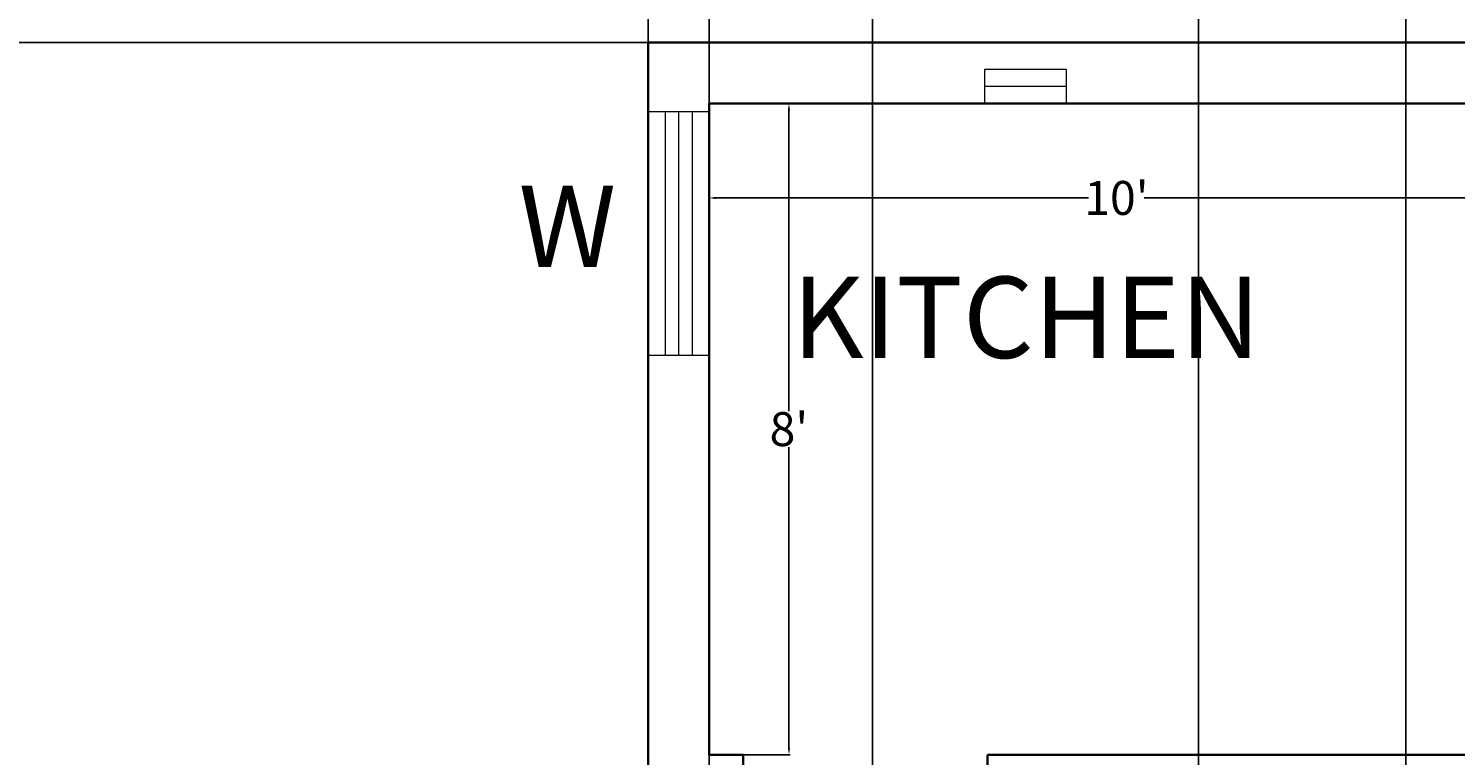
# Model space of a CAD drawing. Units: inches. Extents: x -304 to 580, y 363 to 1149.
# Tile 9 of 11: x -114 to 96, y 900 to 1007. Entities that reach past the tile are written whole.
import ezdxf

# ---------------------------------------------------------------- set-up
doc = ezdxf.new("R2010")
doc.units = ezdxf.units.IN
doc.header["$MEASUREMENT"] = 0
for name, color, linetype, lineweight in [('A-ANNO-DIMS', 2, 'Continuous', 13), ('A-ANNO-IDEN', 7, 'Continuous', 18), ('A-AREA-IDEN', 7, 'Continuous', 25), ('A-GLAZ', 4, 'Continuous', 18), ('A-GLAZ-VENT', 4, 'Continuous', 18), ('A-WALL', 40, 'Continuous', 35)]:
    doc.layers.add(name, color=color, linetype=linetype, lineweight=lineweight)
doc.styles.get("Standard").update_dxf_attribs({"font": 'arial.ttf'})
doc.dimstyles.get("Standard").update_dxf_attribs({"dimtxt": 1, "dimasz": 1, "dimexe": 0.18, "dimexo": 0.0625, "dimgap": 0.09, "dimtad": 0, "dimtih": 1, "dimtoh": 1, "dimdec": 0, "dimzin": 0, "dimdsep": 46, "dimlunit": 3, "dimtxsty": 'Standard', "dimcen": 0.09, "dimadec": 0, "dimazin": 0, "dimtfac": 1, "dimtdec": 0, "dimtofl": 0, "dimtmove": 0, "dimatfit": 3, "dimfxl": 1, "dimtolj": 1, "dimtzin": 0, "dimarcsym": 0})

# ---------------------------------------------------------------- blocks, each defined once
blk = doc.blocks.new('*D1')
at = {"layer": 'A-ANNO-DIMS', "color": 0, "lineweight": -2, "transparency": 16777216}
for p, q in [((-22.63, 1004.95), (-237.62, 1004.95)), ((-237.44, 1003.95), (-237.44, 721.93)), ((-237.44, 402.95), (-237.44, 684.96)), ((-22.63, 401.95), (-237.62, 401.95))]:
    blk.add_line(p, q, dxfattribs=at)
at = {"layer": 'A-ANNO-DIMS', "color": 0, "transparency": 16777216}
for points in [[(-237.61, 1003.95), (-237.28, 1003.95), (-237.44, 1004.95)], [(-237.61, 402.95), (-237.28, 402.95), (-237.44, 401.95)]]:
    blk.add_solid(points, dxfattribs=at)
at = {"layer": 'Defpoints', "color": 0, "transparency": 16777216}
for p in [(-22.57, 1004.95), (-237.44, 401.95), (-22.57, 401.95)]:
    blk.add_point(p, dxfattribs=at)
at = {"layer": 'A-ANNO-DIMS', "color": 0, "transparency": 16777216, "insert": (-237.44, 703.45), "char_height": 1, "attachment_point": 5}
blk.add_mtext('\\A1;{\\H36x;50\'-3"}', dxfattribs=at)
blk = doc.blocks.new('*D2')
at = {"layer": 'A-ANNO-DIMS', "color": 0, "lineweight": -2, "transparency": 16777216}
for p, q in [((-22.57, 1005.01), (-22.57, 1060.38)), ((-21.57, 1060.2), (84.7, 1060.2)), ((315.43, 1060.2), (209.16, 1060.2)), ((316.43, 1005.01), (316.43, 1060.38))]:
    blk.add_line(p, q, dxfattribs=at)
at = {"layer": 'A-ANNO-DIMS', "color": 0, "transparency": 16777216}
for points in [[(-21.57, 1060.37), (-21.57, 1060.04), (-22.57, 1060.2)], [(315.43, 1060.37), (315.43, 1060.04), (316.43, 1060.2)]]:
    blk.add_solid(points, dxfattribs=at)
at = {"layer": 'Defpoints', "color": 0, "transparency": 16777216}
for p in [(316.43, 1060.2), (-22.57, 1004.95), (316.43, 1004.95)]:
    blk.add_point(p, dxfattribs=at)
at = {"layer": 'A-ANNO-DIMS', "color": 0, "transparency": 16777216, "insert": (146.93, 1060.2), "char_height": 1, "attachment_point": 5}
blk.add_mtext('\\A1;{\\H36x;28\'-3"}', dxfattribs=at)
blk = doc.blocks.new('*D5')
at = {"layer": 'A-ANNO-DIMS', "color": 0, "lineweight": -2, "transparency": 16777216}
for p, q in [((-13.57, 995.88), (-13.57, 981.84)), ((106.43, 995.88), (106.43, 981.84)), ((-12.57, 982.02), (42.33, 982.02)), ((105.43, 982.02), (50.53, 982.02))]:
    blk.add_line(p, q, dxfattribs=at)
at = {"layer": 'A-ANNO-DIMS', "color": 0, "transparency": 16777216}
for points in [[(-12.57, 982.19), (-12.57, 981.85), (-13.57, 982.02)], [(105.43, 982.19), (105.43, 981.85), (106.43, 982.02)]]:
    blk.add_solid(points, dxfattribs=at)
at = {"layer": 'Defpoints', "color": 0, "transparency": 16777216}
for p in [(-13.57, 995.95), (106.43, 995.95), (106.43, 982.02)]:
    blk.add_point(p, dxfattribs=at)
at = {"layer": 'A-ANNO-DIMS', "color": 0, "transparency": 16777216, "insert": (46.43, 982.02), "char_height": 1, "attachment_point": 5}
blk.add_mtext("\\A1;{\\H5x;10'}", dxfattribs=at)
blk = doc.blocks.new('*D6')
at = {"layer": 'A-ANNO-DIMS', "color": 0, "lineweight": -2, "transparency": 16777216}
for p, q in [((-13.51, 995.95), (-1.64, 995.95)), ((-1.82, 994.95), (-1.82, 950.59)), ((-1.82, 900.95), (-1.82, 945.3)), ((-13.51, 899.95), (-1.64, 899.95))]:
    blk.add_line(p, q, dxfattribs=at)
at = {"layer": 'A-ANNO-DIMS', "color": 0, "transparency": 16777216}
for points in [[(-1.98, 994.95), (-1.65, 994.95), (-1.82, 995.95)], [(-1.98, 900.95), (-1.65, 900.95), (-1.82, 899.95)]]:
    blk.add_solid(points, dxfattribs=at)
at = {"layer": 'Defpoints', "color": 0, "transparency": 16777216}
for p in [(-13.57, 995.95), (-13.57, 899.95), (-1.82, 899.95)]:
    blk.add_point(p, dxfattribs=at)
at = {"layer": 'A-ANNO-DIMS', "color": 0, "transparency": 16777216, "insert": (-1.82, 947.95), "char_height": 1, "attachment_point": 5}
blk.add_mtext("\\A1;{\\H5x;8'}", dxfattribs=at)
blk = doc.blocks.new('WIN-36IN')
for p, q in [((0, 6.5), (36, 6.5)), ((0, 4.5), (36, 4.5)), ((0, 2.5), (36, 2.5))]:
    blk.add_line(p, q)
blk.add_lwpolyline([(0, 0), (0, 9), (36, 9), (36, 0)], close=True)
blk = doc.blocks.new('VENT-12IN')
blk.add_line((0, 2.5), (12, 2.5))
blk.add_lwpolyline([(0, 0), (0, 5), (12, 5), (12, 0)], close=True)
blk = doc.blocks.new('*D34')
at = {"layer": 'A-ANNO-DIMS', "color": 0, "lineweight": -2, "transparency": 16777216}
for p, q in [((10.51, 550.01), (10.51, 1042.88)), ((11.51, 1042.7), (33.07, 1042.7)), ((57.51, 1042.7), (35.95, 1042.7)), ((58.51, 550.01), (58.51, 1042.88))]:
    blk.add_line(p, q, dxfattribs=at)
at = {"layer": 'A-ANNO-DIMS', "color": 0, "transparency": 16777216}
for points in [[(11.51, 1042.86), (11.51, 1042.53), (10.51, 1042.7)], [(57.51, 1042.86), (57.51, 1042.53), (58.51, 1042.7)]]:
    blk.add_solid(points, dxfattribs=at)
at = {"layer": 'Defpoints', "color": 0, "transparency": 16777216}
for p in [(58.51, 1042.7), (10.51, 549.95), (58.51, 549.95)]:
    blk.add_point(p, dxfattribs=at)
at = {"layer": 'A-ANNO-DIMS', "color": 0, "transparency": 16777216, "insert": (34.51, 1042.7), "char_height": 1, "attachment_point": 5}
blk.add_mtext('\\A1;4\'-0"', dxfattribs=at)
blk = doc.blocks.new('*D35')
at = {"layer": 'A-ANNO-DIMS', "color": 0, "lineweight": -2, "transparency": 16777216}
for p, q in [((-13.57, 550.01), (-13.57, 1042.88)), ((-12.57, 1042.7), (-2.96, 1042.7)), ((9.51, 1042.7), (-0.1, 1042.7)), ((10.51, 550.01), (10.51, 1042.88))]:
    blk.add_line(p, q, dxfattribs=at)
at = {"layer": 'A-ANNO-DIMS', "color": 0, "transparency": 16777216}
for points in [[(-12.57, 1042.86), (-12.57, 1042.53), (-13.57, 1042.7)], [(9.51, 1042.86), (9.51, 1042.53), (10.51, 1042.7)]]:
    blk.add_solid(points, dxfattribs=at)
at = {"layer": 'Defpoints', "color": 0, "transparency": 16777216}
for p in [(10.51, 1042.7), (-13.57, 549.95), (10.51, 549.95)]:
    blk.add_point(p, dxfattribs=at)
at = {"layer": 'A-ANNO-DIMS', "color": 0, "transparency": 16777216, "insert": (-1.53, 1042.7), "char_height": 1, "attachment_point": 5}
blk.add_mtext('\\A1;2\'-0"', dxfattribs=at)
blk = doc.blocks.new('*D36')
at = {"layer": 'A-ANNO-DIMS', "color": 0, "lineweight": -2, "transparency": 16777216}
for p, q in [((-22.57, 516.57), (-22.57, 1042.88)), ((-21.57, 1042.7), (30.65, 1042.7)), ((88.04, 1042.7), (35.82, 1042.7)), ((89.04, 516.57), (89.04, 1042.88))]:
    blk.add_line(p, q, dxfattribs=at)
at = {"layer": 'A-ANNO-DIMS', "color": 0, "transparency": 16777216}
for points in [[(-21.57, 1042.86), (-21.57, 1042.53), (-22.57, 1042.7)], [(88.04, 1042.86), (88.04, 1042.53), (89.04, 1042.7)]]:
    blk.add_solid(points, dxfattribs=at)
at = {"layer": 'Defpoints', "color": 0, "transparency": 16777216}
for p in [(89.04, 1042.7), (-22.57, 516.51), (89.04, 516.51)]:
    blk.add_point(p, dxfattribs=at)
at = {"layer": 'A-ANNO-DIMS', "color": 0, "transparency": 16777216, "insert": (33.23, 1042.7), "char_height": 1, "attachment_point": 5}
blk.add_mtext('\\A1;9\'-3 1/2"', dxfattribs=at)

msp = doc.modelspace()

# ---------------------------------------------------------------- linework, layer by layer
at = {"layer": 'A-WALL'}
for p, q in [((-22.57, 1004.95), (316.43, 1004.95)), ((-22.57, 516.51), (-22.57, 1004.95)), ((-13.57, 995.95), (106.43, 995.95)), ((-13.57, 899.95), (-13.57, 995.95)), ((-13.57, 899.95), (-8.57, 899.95)), ((-8.57, 899.95), (-8.57, 894.95)), ((27.43, 899.95), (27.43, 894.95)), ((27.43, 899.95), (106.43, 899.95))]:
    msp.add_line(p, q, dxfattribs=at)

# ---------------------------------------------------------------- block references
at = {"layer": 'A-GLAZ', "rotation": 270}
msp.add_blockref('WIN-36IN', (-22.57, 994.78), dxfattribs=at)
at = {"layer": 'A-GLAZ-VENT'}
msp.add_blockref('VENT-12IN', (27.04, 995.98), dxfattribs=at)

# ---------------------------------------------------------------- texts
at = {"layer": 'A-ANNO-IDEN', "insert": (-41.64, 983.83), "char_height": 12, "attachment_point": 1}
msp.add_mtext_dynamic_manual_height_columns('W', width=41.6501, gutter_width=1, heights=[0], dxfattribs=at)
at = {"layer": 'A-AREA-IDEN', "insert": (-1.37, 970.42), "char_height": 12, "attachment_point": 1}
msp.add_mtext_dynamic_manual_height_columns('KITCHEN', width=79.7399, gutter_width=1, heights=[0], dxfattribs=at)

# ---------------------------------------------------------------- dimensions: what is measured, and where the dimension line sits
at = {"layer": 'A-ANNO-DIMS'}
for base, p1, p2, text, picture, middle in [((316.43, 1060.2), (-22.57, 1004.95), (316.43, 1004.95), '{\\H36x;<>}', '*D2', (146.93, 1060.2)), ((106.43, 982.02), (-13.57, 995.95), (106.43, 995.95), '{\\H5x;<>}', '*D5', (46.43, 982.02))]:
    dim = msp.add_linear_dim(base=base, p1=p1, p2=p2, text=text, dimstyle='Standard', override={"dimclrd": 0, "dimclre": 0, "dimclrt": 0}, dxfattribs=at)
    dim.commit()
    dim.dimension.update_dxf_attribs({"geometry": picture, "text_midpoint": middle})
for base, p1, p2, picture, middle in [((89.04, 1042.7), (-22.57, 516.51), (89.04, 516.51), '*D36', (33.23, 1042.7)), ((10.51, 1042.7), (-13.57, 549.95), (10.51, 549.95), '*D35', (-1.53, 1042.7)), ((58.51, 1042.7), (10.51, 549.95), (58.51, 549.95), '*D34', (34.51, 1042.7))]:
    dim = msp.add_linear_dim(base=base, p1=p1, p2=p2, dimstyle='Standard', override={"dimdec": 1, "dimlfac": 1, "dimrnd": 0, "dimzin": 1, "dimdsep": 46, "dimlunit": 4, "dimfrac": 2}, dxfattribs=at)
    dim.commit()
    dim.dimension.update_dxf_attribs({"geometry": picture, "text_midpoint": middle})
for base, p1, p2, text, picture, middle in [((-237.44, 401.95), (-22.57, 1004.95), (-22.57, 401.95), '{\\H36x;<>}', '*D1', (-237.44, 703.45)), ((-1.82, 899.95), (-13.57, 995.95), (-13.57, 899.95), '{\\H5x;<>}', '*D6', (-1.82, 947.95))]:
    dim = msp.add_linear_dim(base=base, p1=p1, p2=p2, angle=90, text=text, dimstyle='Standard', override={"dimclrd": 0, "dimclre": 0, "dimclrt": 0}, dxfattribs=at)
    dim.commit()
    dim.dimension.update_dxf_attribs({"geometry": picture, "text_midpoint": middle})

doc.saveas('drawing.dxf')
